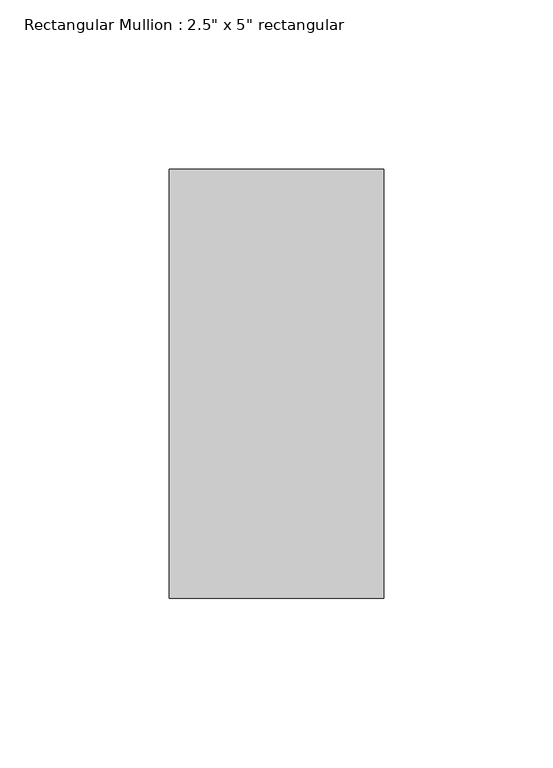
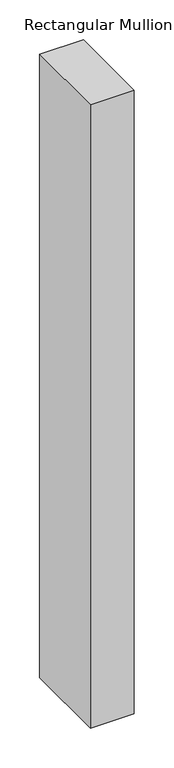
"""IFC4 building model written with IfcOpenShell, lengths in millimetres: member geometry."""

from ifc_helpers import new_model, si_unit, frame, origin, place, context, project, spatial, polyline, outline, extrude, source, transform, mapped, element, save


def member_6e66df9c(model_context):
    return source(origin(), model_context, "Body", "SweptSolid", [
        extrude(outline(polyline([(0.0, 63.5), (0.0, -63.5), (-63.5, -63.5), (-63.5, 63.5), (0.0, 63.5)])), frame((0.0, 0.0, -953.65), z_axis=(0.0, 0.0, 1.0), x_axis=(1.0, 0.0, 0.0)), (0.0, 0.0, 1.0), 953.65),
    ])


if __name__ == "__main__":
    model = new_model("IFC4")
    model_context = context("Model", 3, world=origin())
    ifc_project = project(units=[si_unit("LENGTHUNIT", "METRE", prefix="MILLI")], contexts=[model_context])
    site = spatial("IfcSite", under=ifc_project)
    building = spatial("IfcBuilding", under=site)
    placement = place(None, origin())
    member_shape = member_6e66df9c(model_context)
    element("IfcMember", 1, ObjectType="Rectangular Mullion : 2.5\" x 5\" rectangular", at=placement, inside=building, context=model_context, shape_type="MappedRepresentation", body=[
        mapped(member_shape, transform((0.0, 0.0, 0.0), x_axis=(1.0, 0.0, 0.0), y_axis=(0.0, 1.0, 0.0), z_axis=(0.0, 0.0, 1.0))),
    ])
    save(model, "model.ifc")

# Revit data of these elements
# Type "Rectangular Mullion : 2.5\" x 5\" rectangular"
#   built-in parameter 1007304 = 0.416667 (stored number, unit not read)
#   built-in parameter 1007301 = 0.104167 (stored number, unit not read)
#   built-in parameter 1007300 = 0.104167 (stored number, unit not read)
# Element 1 (IfcMember, "Rectangular Mullion : 2.5\" x 5\" rectangular")
#   Materials on its faces: "Damp-proofing"
# Materials
#   "Damp-proofing": class "Generic", colour RGB 127 127 127, transparency 0, Description = "Damp-proofing", Cost = 0
